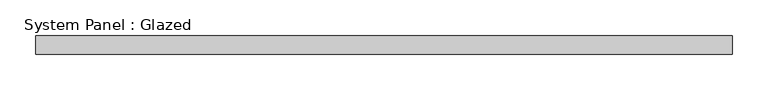
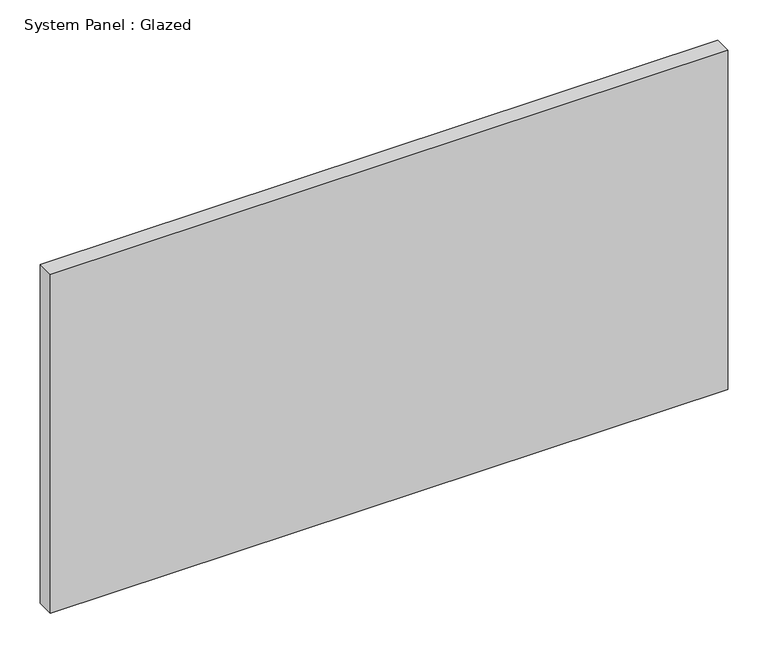
"""IFC4 building model written with IfcOpenShell, lengths in millimetres: plate geometry, System Panel : Glazed."""

from ifc_helpers import new_model, si_unit, origin, origin_with_axes, place, context, project, spatial, polyline, outline, extrude, source, transform, mapped, element, save


def system_panel_glazed_b5d2153e(model_context):
    return source(origin(), model_context, "Body", "SweptSolid", [
        extrude(outline(polyline([(485.7750001, 19.05), (-485.7750001, 19.05), (-485.7750001, 44.45), (485.7750001, 44.45), (485.7750001, 19.05)])), origin_with_axes(), (0.0, 0.0, 1.0), 514.35),
    ])


if __name__ == "__main__":
    model = new_model("IFC4")
    model_context = context("Model", 3, world=origin())
    ifc_project = project(units=[si_unit("LENGTHUNIT", "METRE", prefix="MILLI")], contexts=[model_context])
    site = spatial("IfcSite", under=ifc_project)
    building = spatial("IfcBuilding", under=site)
    placement = place(None, origin())
    system_panel_glazed_shape = system_panel_glazed_b5d2153e(model_context)
    element("IfcPlate", 1, ObjectType="System Panel : Glazed", at=placement, inside=building, context=model_context, shape_type="MappedRepresentation", body=[
        mapped(system_panel_glazed_shape, transform((0.0, 0.0, 0.0), x_axis=(1.0, 0.0, 0.0), y_axis=(0.0, 1.0, 0.0), z_axis=(0.0, 0.0, 1.0))),
    ])
    save(model, "model.ifc")

# Revit data of these elements
# Type "System Panel : Glazed"
#   Construction Type Id = "GSP4R"
#   Analytic Construction = "1/8 in Pilkington single glazing"
#   Visual Light Transmittance = 0.9
#   Solar Heat Gain Coefficient = 0.86
#   Heat Transfer Coefficient (U) = 1.18115 BTU/(h·ft²·°F)
#   Define Thermal Properties by = 1
# Element 1 (IfcPlate, "System Panel : Glazed")
#   Materials on its faces: "Glass"
# Materials
#   "Glass": class "Glass", colour RGB 0 128 192, transparency 0.75, Description = "Soda Lime Glass", Cost = 0
